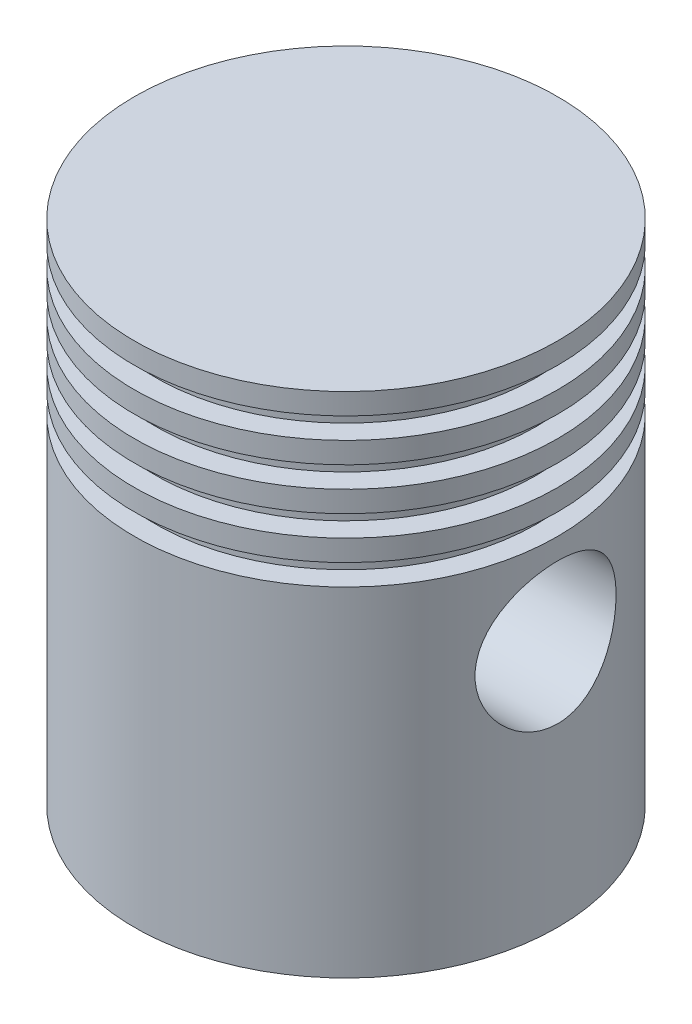
SolidWorks part; units mm, degrees
material "Plain Carbon Steel"
ref_plane "Front Plane" through (0, 0, 0) normal (0, 0, 1) x (1, 0, 0)
ref_plane "Top Plane" through (0, 0, 0) normal (0, 1, 0) x (1, 0, 0)
ref_plane "Right Plane" through (0, 0, 0) normal (1, 0, 0) x (0, 0, -1)
sketch "Piston Profile Sketch" plane through (0, 0, 0) normal (0, 0, 1) x (1, 0, 0)
  line L0 (0, 71.8701) -> (0, 60) construction
  line L1 (-24, 0) -> (-30, 0)
  line L2 (-30, 0) -> (-30, 48)
  line L3 (-30, 48) -> (-27, 48)
  line L4 (-27, 48) -> (-27, 51)
  line L5 (-27, 51) -> (-30, 51)
  line L6 (-30, 51) -> (-30, 54)
  line L7 (-30, 54) -> (-27, 54)
  line L8 (-27, 54) -> (-27, 57)
  line L9 (-27, 57) -> (-30, 57)
  line L10 (-30, 57) -> (-30, 60)
  line L11 (-30, 60) -> (-27, 60)
  line L12 (-27, 60) -> (-27, 63)
  line L13 (-27, 63) -> (-30, 63)
  line L14 (-30, 63) -> (-30, 66)
  line L15 (-30, 66) -> (-27, 66)
  line L16 (-27, 66) -> (-27, 69)
  line L17 (-27, 69) -> (-30, 69)
  line L18 (-30, 69) -> (-30, 72)
  line L19 (-30, 72) -> (0, 72)
  line L21 (-24, 60) -> (0, 60)
  line L22 (0, 60) -> (0, 72)
  line L23 (0, 0) -> (0, 103.2942) construction
  line L24 (-24, 60) -> (-24, 48)
  line L25 (-24, 48) -> (-10, 48)
  line L26 (-10, 48) -> (-10, 22)
  line L27 (-10, 22) -> (-24, 22)
  line L28 (-24, 22) -> (-24, 0)
  line L29 (0, 35) -> (-84.8301, 35) construction
  dimension "D1" = 72
  dimension "D2" = 30
  dimension "D3" = 24
  dimension "D4" = 3
  dimension "D5" = 3
  dimension "D6" = 3
  dimension "D7" = 12
  dimension "D8" = 10
  dimension "D9" = 26
  dimension "D10" = 22
  dimension "D11" = 35
revolve "Piston Body Revolve" add sketch "Piston Profile Sketch" angle 360 about L22
sketch "Pin Bore Sketch" plane through (0, 0, 0) normal (1, 0, 0) x (0, 0, -1)
  line L0 (0, 0) -> (0, 114.8376) construction
  line L1 (-30, 0) -> (30, 0) construction
  circle A0 centre (0, 35) radius 10
  dimension "D1" = 20
  dimension "D2" = 35
extrude "Gudgeon Pin Bore Ø20" cut sketch "Pin Bore Sketch" against normal mid plane 132
chamfer "Edge Chamfer 2x45°" distance 2 angle 45 1 edges at (24, 0, 0)
sketch "Inner Cavity Sketch" plane through (0, 0, 0) normal (0, -1, 0) x (1, 0, 0)
  line L1 (-10, -14.5) -> (10, -14.5)
  line L2 (-10, -14.5) -> (-10, 14.5)
  line L3 (-10, 14.5) -> (10, 14.5)
  line L4 (10, -14.5) -> (10, 14.5)
  line L5 (-10, -14.5) -> (10, 14.5) construction
  line L6 (-10, 14.5) -> (10, -14.5) construction
  point P0 (0, 0)
  dimension "D1" = 20
  dimension "D2" = 29
extrude "Inner Cavity Cut" cut sketch "Inner Cavity Sketch" against normal blind 48
